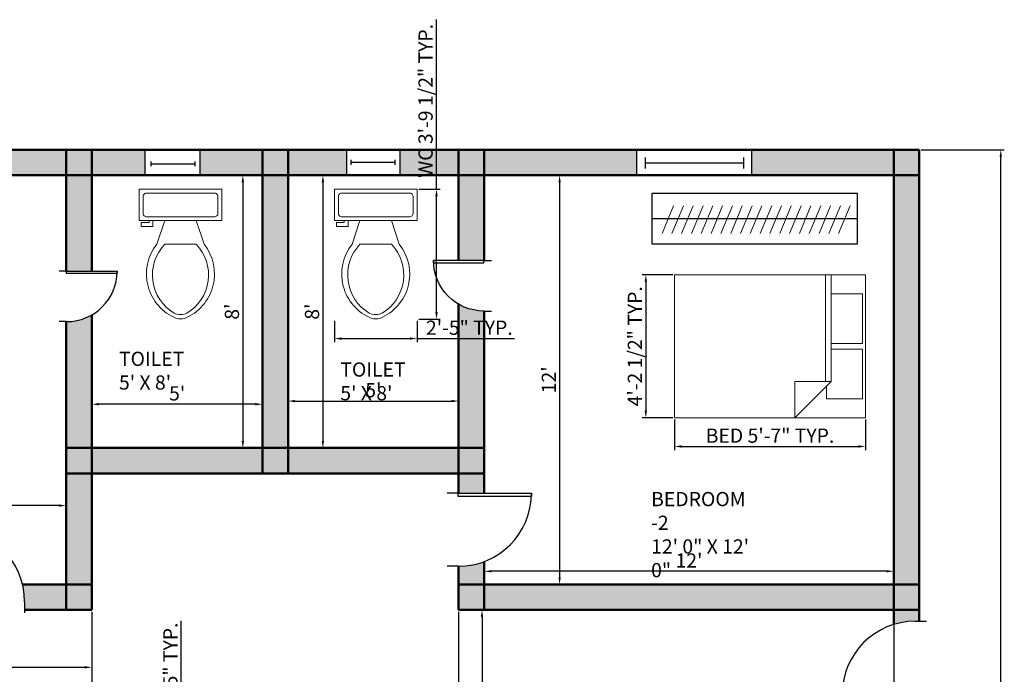
# Model space of a CAD drawing. Units: millimetres. Extents: x 2829 to 4029, y 962 to 1687.
# Tile 4 of 7: x 3053 to 3399, y 1440 to 1670. Entities that reach past the tile are written whole.
import ezdxf

# ---------------------------------------------------------------- set-up
doc = ezdxf.new("R2010")
doc.units = ezdxf.units.MM
for name, color, linetype, lineweight in [('A-ANNO-DIMS', 140, 'Continuous', 18), ('A-AREA-IDEN', 190, 'Continuous', 25), ('A-FLOR-CASE', 90, 'Continuous', 25), ('A-FLOR-CASE-PATT', 90, 'Continuous', 13), ('A-FLOR-FIXT', 90, 'Continuous', 18), ('A-WALL-PATT', 2, 'Continuous', 13), ('doors', 10, 'Continuous', 25), ('furniture', 90, 'Continuous', 18), ('walls', 50, 'Continuous', 50), ('windows', 30, 'Continuous', 25)]:
    doc.layers.add(name, color=color, linetype=linetype, lineweight=lineweight)
doc.styles.get("Standard").update_dxf_attribs({"font": 'arial.ttf'})
doc.dimstyles.new('ISO-25', dxfattribs={"dimtxt": 5, "dimasz": 2.5, "dimexe": 1.25, "dimexo": 0.625, "dimtad": 1, "dimdec": 0, "dimlunit": 3, "dimtxsty": 'Standard', "dimcen": 2.5, "dimadec": 0, "dimazin": 0, "dimtfac": 1, "dimtdec": 0, "dimtmove": 0, "dimatfit": 3, "dimfxl": 1, "dimarcsym": 0})

# ---------------------------------------------------------------- blocks, each defined once
blk = doc.blocks.new('*U2')
for p, q in [((0, 0), (0, -6)), ((40, 0), (40, -6))]:
    blk.add_line(p, q)
blk.add_lwpolyline([(0, 0), (0, 40), (1.75, 40), (1.75, 0)], close=True)
blk.add_arc((0, 0), 40, 0, 90)
blk = doc.blocks.new('*U5')
for p, q in [((0, 4), (0, 0)), ((0, 2), (36, 2)), ((36, 4), (36, 0))]:
    blk.add_line(p, q)
blk = doc.blocks.new('*U4')
for p, q in [((0, 4), (0, 0)), ((36, 4), (36, 0)), ((0, 2), (36, 2))]:
    blk.add_line(p, q)
blk = doc.blocks.new('Bed - Queen')
for p, q in [((0, -80.00003), (0, 0)), ((0, 0), (59.99999, 0)), ((59.99999, 0), (59.99999, -80.00003)), ((7.99999, -1.2), (28.79998, -1.2)), ((7.99999, -14.4), (7.99999, -1.2)), ((28.79998, -1.2), (28.79998, -14.4)), ((31.19999, -1.2), (51.99999, -1.2)), ((31.19999, -14.4), (31.19999, -1.2)), ((51.99999, -1.2), (51.99999, -16.4)), ((0, -14.4), (44.8, -14.4)), ((59.99999, -29.6), (44.8, -14.4)), ((44.8, -14.4), (44.8, -29.6)), ((51.99999, -16.4), (46.79936, -16.4)), ((44.8, -16.8), (0, -16.8)), ((44.8, -29.6), (59.99999, -29.6)), ((59.99999, -80.00003), (0, -80.00003))]:
    blk.add_line(p, q)
blk = doc.blocks.new('Toilet - top')
for p, q in [((9.5, -6), (9.5, -2)), ((-10, -8.5), (-8, -8.5)), ((-10, -9.5), (-10, -8.5)), ((-7, -9.5), (-10, -9.5)), ((-8, -8.5), (-8, -8)), ((-7, -8), (-7, -9.5)), ((-4, -8), (-6, -14)), ((4, -8), (6, -14)), ((4, -14), (-4, -14))]:
    blk.add_line(p, q)
blk.add_lwpolyline([(10.5, -8), (10.5, 0), (-10.5, 0), (-10.5, -8)], close=True)
for points in [[(-9.5, -2), (-9.5, -6)], [(8.5, -1), (-8.5, -1)], [(-8.5, -7), (8.5, -7)]]:
    blk.add_lwpolyline(points)
for centre, radius, start, end in [((-8.62, -1.88), 0.884, 81.8699, 188.1301), ((8.62, -1.88), 0.884, 351.8699, 98.1301), ((-8.62, -6.12), 0.884, 171.8699, 278.1301), ((8.62, -6.12), 0.884, 261.8699, 8.1301), ((3.52, -21.58), 12.17, 141.4691, 247.9714), ((4.2, -21.82), 11.33, 136.3677, 238.9468), ((-3.52, -21.58), 12.17, 292.0284, 38.5307), ((-4.2, -21.82), 11.33, 301.053, 43.6321), ((0, -27.88), 4, 245.7318, 294.2682), ((0, -29), 4, 254.8605, 285.1395)]:
    blk.add_arc(centre, radius, start, end)
blk = doc.blocks.new('*D12')
at = {"layer": 'A-ANNO-DIMS', "color": 0, "lineweight": -2, "transparency": 16777216}
for p, q in [((2937.31, 1499.73), (2937.31, 1500.36)), ((3069.31, 1499.73), (3069.31, 1500.36)), ((3066.81, 1499.11), (2939.81, 1499.11))]:
    blk.add_line(p, q, dxfattribs=at)
at = {"layer": 'A-ANNO-DIMS', "color": 0, "transparency": 16777216}
for points in [[(2939.81, 1499.52), (2939.81, 1498.69), (2937.31, 1499.11)], [(3066.81, 1499.52), (3066.81, 1498.69), (3069.31, 1499.11)]]:
    blk.add_solid(points, dxfattribs=at)
at = {"layer": 'Defpoints', "color": 0, "transparency": 16777216}
for p in [(2937.31, 1499.11), (2937.31, 1499.11), (3069.31, 1499.11)]:
    blk.add_point(p, dxfattribs=at)
at = {"layer": 'A-ANNO-DIMS', "color": 0, "transparency": 16777216, "insert": (3003.31, 1502.24), "char_height": 5, "attachment_point": 5}
blk.add_mtext("11'", dxfattribs=at)
blk = doc.blocks.new('*D13')
at = {"layer": 'A-ANNO-DIMS', "color": 0, "lineweight": -2, "transparency": 16777216}
for p, q in [((3131.71, 1615.38), (3132.65, 1615.38)), ((3131.4, 1612.88), (3131.4, 1521.88)), ((3131.71, 1519.38), (3132.65, 1519.38))]:
    blk.add_line(p, q, dxfattribs=at)
at = {"layer": 'A-ANNO-DIMS', "color": 0, "transparency": 16777216}
for points in [[(3130.98, 1612.88), (3131.82, 1612.88), (3131.4, 1615.38)], [(3130.98, 1521.88), (3131.82, 1521.88), (3131.4, 1519.38)]]:
    blk.add_solid(points, dxfattribs=at)
at = {"layer": 'Defpoints', "color": 0, "transparency": 16777216}
for p in [(3131.09, 1615.38), (3131.09, 1519.38), (3131.4, 1519.38)]:
    blk.add_point(p, dxfattribs=at)
at = {"layer": 'A-ANNO-DIMS', "color": 0, "transparency": 16777216, "insert": (3128.22, 1567.38), "char_height": 5, "attachment_point": 5, "rotation": 90}
blk.add_mtext("8'", dxfattribs=at)
blk = doc.blocks.new('*D14')
at = {"layer": 'A-ANNO-DIMS', "color": 0, "lineweight": -2, "transparency": 16777216}
for p, q in [((3078.31, 1535.41), (3078.31, 1536.04)), ((3135.81, 1534.79), (3080.81, 1534.79)), ((3138.31, 1535.41), (3138.31, 1536.04))]:
    blk.add_line(p, q, dxfattribs=at)
at = {"layer": 'A-ANNO-DIMS', "color": 0, "transparency": 16777216}
for points in [[(3080.81, 1535.2), (3080.81, 1534.37), (3078.31, 1534.79)], [(3135.81, 1535.2), (3135.81, 1534.37), (3138.31, 1534.79)]]:
    blk.add_solid(points, dxfattribs=at)
at = {"layer": 'Defpoints', "color": 0, "transparency": 16777216}
for p in [(3078.31, 1534.79), (3078.31, 1534.79), (3138.31, 1534.79)]:
    blk.add_point(p, dxfattribs=at)
at = {"layer": 'A-ANNO-DIMS', "color": 0, "transparency": 16777216, "insert": (3108.31, 1537.95), "char_height": 5, "attachment_point": 5}
blk.add_mtext("5'", dxfattribs=at)
blk = doc.blocks.new('*D15')
at = {"layer": 'A-ANNO-DIMS', "color": 0, "lineweight": -2, "transparency": 16777216}
for p, q in [((3147.31, 1535.41), (3147.31, 1537.14)), ((3149.81, 1535.89), (3204.81, 1535.89)), ((3207.31, 1535.41), (3207.31, 1537.14))]:
    blk.add_line(p, q, dxfattribs=at)
at = {"layer": 'A-ANNO-DIMS', "color": 0, "transparency": 16777216}
for points in [[(3149.81, 1536.31), (3149.81, 1535.47), (3147.31, 1535.89)], [(3204.81, 1536.31), (3204.81, 1535.47), (3207.31, 1535.89)]]:
    blk.add_solid(points, dxfattribs=at)
at = {"layer": 'Defpoints', "color": 0, "transparency": 16777216}
for p in [(3147.31, 1534.79), (3207.31, 1535.89), (3207.31, 1534.79)]:
    blk.add_point(p, dxfattribs=at)
at = {"layer": 'A-ANNO-DIMS', "color": 0, "transparency": 16777216, "insert": (3177.31, 1539.06), "char_height": 5, "attachment_point": 5}
blk.add_mtext("5'", dxfattribs=at)
blk = doc.blocks.new('*D16')
at = {"layer": 'A-ANNO-DIMS', "color": 0, "lineweight": -2, "transparency": 16777216}
for p, q in [((3155.72, 1615.38), (3160.81, 1615.38)), ((3159.56, 1612.88), (3159.56, 1521.88)), ((3155.72, 1519.38), (3160.81, 1519.38))]:
    blk.add_line(p, q, dxfattribs=at)
at = {"layer": 'A-ANNO-DIMS', "color": 0, "transparency": 16777216}
for points in [[(3159.15, 1612.88), (3159.98, 1612.88), (3159.56, 1615.38)], [(3159.15, 1521.88), (3159.98, 1521.88), (3159.56, 1519.38)]]:
    blk.add_solid(points, dxfattribs=at)
at = {"layer": 'Defpoints', "color": 0, "transparency": 16777216}
for p in [(3155.1, 1615.38), (3155.1, 1519.38), (3159.56, 1519.38)]:
    blk.add_point(p, dxfattribs=at)
at = {"layer": 'A-ANNO-DIMS', "color": 0, "transparency": 16777216, "insert": (3156.39, 1567.38), "char_height": 5, "attachment_point": 5, "rotation": 90}
blk.add_mtext("8'", dxfattribs=at)
blk = doc.blocks.new('*D17')
at = {"layer": 'A-ANNO-DIMS', "color": 0, "lineweight": -2, "transparency": 16777216}
for p, q in [((3360.31, 1480.59), (3360.31, 1474.74)), ((3216.31, 1476.61), (3216.31, 1477.24)), ((3357.81, 1475.99), (3218.81, 1475.99))]:
    blk.add_line(p, q, dxfattribs=at)
at = {"layer": 'A-ANNO-DIMS', "color": 0, "transparency": 16777216}
for points in [[(3218.81, 1476.4), (3218.81, 1475.57), (3216.31, 1475.99)], [(3357.81, 1476.4), (3357.81, 1475.57), (3360.31, 1475.99)]]:
    blk.add_solid(points, dxfattribs=at)
at = {"layer": 'Defpoints', "color": 0, "transparency": 16777216}
for p in [(3360.31, 1481.22), (3216.31, 1475.99), (3216.31, 1475.99)]:
    blk.add_point(p, dxfattribs=at)
at = {"layer": 'A-ANNO-DIMS', "color": 0, "transparency": 16777216, "insert": (3288.31, 1479.12), "char_height": 5, "attachment_point": 5}
blk.add_mtext("12'", dxfattribs=at)
blk = doc.blocks.new('*D18')
at = {"layer": 'A-ANNO-DIMS', "color": 0, "lineweight": -2, "transparency": 16777216}
for p, q in [((3243.44, 1615.38), (3244.06, 1615.38)), ((3242.81, 1612.88), (3242.81, 1473.88)), ((3243.44, 1471.38), (3244.06, 1471.38))]:
    blk.add_line(p, q, dxfattribs=at)
at = {"layer": 'A-ANNO-DIMS', "color": 0, "transparency": 16777216}
for points in [[(3242.4, 1612.88), (3243.23, 1612.88), (3242.81, 1615.38)], [(3242.4, 1473.88), (3243.23, 1473.88), (3242.81, 1471.38)]]:
    blk.add_solid(points, dxfattribs=at)
at = {"layer": 'Defpoints', "color": 0, "transparency": 16777216}
for p in [(3242.81, 1615.38), (3242.81, 1471.38), (3242.81, 1471.38)]:
    blk.add_point(p, dxfattribs=at)
at = {"layer": 'A-ANNO-DIMS', "color": 0, "transparency": 16777216, "insert": (3239.68, 1543.38), "char_height": 5, "attachment_point": 5, "rotation": 90}
blk.add_mtext("12'", dxfattribs=at)
blk = doc.blocks.new('*D27')
at = {"layer": 'A-ANNO-DIMS', "color": 0, "lineweight": -2, "transparency": 16777216}
for p, q in [((2937.31, 1461.76), (2937.31, 1440.93)), ((3078.31, 1461.76), (3078.31, 1440.93)), ((2939.81, 1442.18), (3075.81, 1442.18))]:
    blk.add_line(p, q, dxfattribs=at)
at = {"layer": 'A-ANNO-DIMS', "color": 0, "transparency": 16777216}
for points in [[(2939.81, 1442.59), (2939.81, 1441.76), (2937.31, 1442.18)], [(3075.81, 1442.59), (3075.81, 1441.76), (3078.31, 1442.18)]]:
    blk.add_solid(points, dxfattribs=at)
at = {"layer": 'Defpoints', "color": 0, "transparency": 16777216}
for p in [(2937.31, 1462.38), (3078.31, 1462.38), (3078.31, 1442.18)]:
    blk.add_point(p, dxfattribs=at)
at = {"layer": 'A-ANNO-DIMS', "color": 0, "transparency": 16777216, "insert": (3007.81, 1445.36), "char_height": 5, "attachment_point": 5}
blk.add_mtext('11\'-9"', dxfattribs=at)
blk = doc.blocks.new('*D28')
at = {"layer": 'A-ANNO-DIMS', "color": 0, "lineweight": -2, "transparency": 16777216}
for p, q in [((3215.69, 1462.38), (3214.27, 1462.38)), ((3215.52, 1459.88), (3215.52, 1326.88)), ((3215.69, 1324.38), (3214.27, 1324.38))]:
    blk.add_line(p, q, dxfattribs=at)
at = {"layer": 'A-ANNO-DIMS', "color": 0, "transparency": 16777216}
for points in [[(3215.1, 1459.88), (3215.93, 1459.88), (3215.52, 1462.38)], [(3215.1, 1326.88), (3215.93, 1326.88), (3215.52, 1324.38)]]:
    blk.add_solid(points, dxfattribs=at)
at = {"layer": 'Defpoints', "color": 0, "transparency": 16777216}
for p in [(3216.31, 1462.38), (3215.52, 1324.38), (3216.31, 1324.38)]:
    blk.add_point(p, dxfattribs=at)
at = {"layer": 'A-ANNO-DIMS', "color": 0, "transparency": 16777216, "insert": (3212.34, 1393.38), "char_height": 5, "attachment_point": 5, "rotation": 90}
blk.add_mtext('11\'-6"', dxfattribs=at)
blk = doc.blocks.new('*D29')
at = {"layer": 'A-ANNO-DIMS', "color": 0, "lineweight": -2, "transparency": 16777216}
for p, q in [((3207.31, 1461.76), (3207.31, 1408.16)), ((3360.31, 1461.76), (3360.31, 1408.16)), ((3209.81, 1409.41), (3357.81, 1409.41))]:
    blk.add_line(p, q, dxfattribs=at)
at = {"layer": 'A-ANNO-DIMS', "color": 0, "transparency": 16777216}
for points in [[(3209.81, 1409.83), (3209.81, 1408.99), (3207.31, 1409.41)], [(3357.81, 1409.83), (3357.81, 1408.99), (3360.31, 1409.41)]]:
    blk.add_solid(points, dxfattribs=at)
at = {"layer": 'Defpoints', "color": 0, "transparency": 16777216}
for p in [(3207.31, 1462.38), (3360.31, 1462.38), (3360.31, 1409.41)]:
    blk.add_point(p, dxfattribs=at)
at = {"layer": 'A-ANNO-DIMS', "color": 0, "transparency": 16777216, "insert": (3283.81, 1412.59), "char_height": 5, "attachment_point": 5}
blk.add_mtext('12\'-9"', dxfattribs=at)
blk = doc.blocks.new('*D30')
at = {"layer": 'A-ANNO-DIMS', "color": 0, "lineweight": -2, "transparency": 16777216}
for p, q in [((3078.31, 1461.76), (3078.31, 1406.92)), ((3207.31, 1461.76), (3207.31, 1406.92)), ((3080.81, 1408.17), (3204.81, 1408.17))]:
    blk.add_line(p, q, dxfattribs=at)
at = {"layer": 'A-ANNO-DIMS', "color": 0, "transparency": 16777216}
for points in [[(3080.81, 1408.59), (3080.81, 1407.75), (3078.31, 1408.17)], [(3204.81, 1408.59), (3204.81, 1407.75), (3207.31, 1408.17)]]:
    blk.add_solid(points, dxfattribs=at)
at = {"layer": 'Defpoints', "color": 0, "transparency": 16777216}
for p in [(3078.31, 1462.38), (3207.31, 1462.38), (3207.31, 1408.17)]:
    blk.add_point(p, dxfattribs=at)
at = {"layer": 'A-ANNO-DIMS', "color": 0, "transparency": 16777216, "insert": (3142.81, 1411.35), "char_height": 5, "attachment_point": 5}
blk.add_mtext('10\'-9"', dxfattribs=at)
blk = doc.blocks.new('*D69')
at = {"layer": 'A-ANNO-DIMS', "color": 0, "lineweight": -2, "transparency": 16777216}
for p, q in [((3283.22, 1529.36), (3283.22, 1518.66)), ((3350.4, 1529.36), (3350.4, 1518.66)), ((3285.72, 1519.91), (3347.9, 1519.91))]:
    blk.add_line(p, q, dxfattribs=at)
at = {"layer": 'A-ANNO-DIMS', "color": 0, "transparency": 16777216}
for points in [[(3285.72, 1520.33), (3285.72, 1519.49), (3283.22, 1519.91)], [(3347.9, 1520.33), (3347.9, 1519.49), (3350.4, 1519.91)]]:
    blk.add_solid(points, dxfattribs=at)
at = {"layer": 'Defpoints', "color": 0, "transparency": 16777216}
for p in [(3283.22, 1529.99), (3350.4, 1529.99), (3350.4, 1519.91)]:
    blk.add_point(p, dxfattribs=at)
at = {"layer": 'A-ANNO-DIMS', "color": 0, "transparency": 16777216, "insert": (3316.81, 1523.08), "char_height": 5, "attachment_point": 5}
blk.add_mtext('BED 5\'-7" TYP.', dxfattribs=at)
blk = doc.blocks.new('*D70')
at = {"layer": 'A-ANNO-DIMS', "color": 0, "lineweight": -2, "transparency": 16777216}
for p, q in [((3282.59, 1580.38), (3271.89, 1580.38)), ((3273.14, 1577.88), (3273.14, 1532.49)), ((3282.59, 1529.99), (3271.89, 1529.99))]:
    blk.add_line(p, q, dxfattribs=at)
at = {"layer": 'A-ANNO-DIMS', "color": 0, "transparency": 16777216}
for points in [[(3272.72, 1577.88), (3273.55, 1577.88), (3273.14, 1580.38)], [(3272.72, 1532.49), (3273.55, 1532.49), (3273.14, 1529.99)]]:
    blk.add_solid(points, dxfattribs=at)
at = {"layer": 'Defpoints', "color": 0, "transparency": 16777216}
for p in [(3283.22, 1580.38), (3273.14, 1529.99), (3283.22, 1529.99)]:
    blk.add_point(p, dxfattribs=at)
at = {"layer": 'A-ANNO-DIMS', "color": 0, "transparency": 16777216, "insert": (3269.93, 1555.18), "char_height": 5, "attachment_point": 5, "rotation": 90}
blk.add_mtext('4\'-2 1/2" TYP.', dxfattribs=at)
blk = doc.blocks.new('*D73')
at = {"layer": 'A-ANNO-DIMS', "color": 0, "lineweight": -2, "transparency": 16777216}
for p, q in [((3199.53, 1610.48), (3199.53, 1670.15)), ((3193.29, 1610.48), (3200.78, 1610.48)), ((3199.53, 1567.25), (3199.53, 1607.98)), ((3193.29, 1564.75), (3200.78, 1564.75))]:
    blk.add_line(p, q, dxfattribs=at)
at = {"layer": 'A-ANNO-DIMS', "color": 0, "transparency": 16777216}
for points in [[(3199.11, 1607.98), (3199.94, 1607.98), (3199.53, 1610.48)], [(3199.11, 1567.25), (3199.94, 1567.25), (3199.53, 1564.75)]]:
    blk.add_solid(points, dxfattribs=at)
at = {"layer": 'Defpoints', "color": 0, "transparency": 16777216}
for p in [(3192.67, 1610.48), (3199.53, 1610.48), (3192.67, 1564.75)]:
    blk.add_point(p, dxfattribs=at)
at = {"layer": 'A-ANNO-DIMS', "color": 0, "transparency": 16777216, "insert": (3196.32, 1641.56), "char_height": 5, "attachment_point": 5, "rotation": 90}
blk.add_mtext('WC 3\'-9 1/2" TYP.', dxfattribs=at)
blk = doc.blocks.new('*D74')
at = {"layer": 'A-ANNO-DIMS', "color": 0, "lineweight": -2, "transparency": 16777216}
for p, q in [((3163.61, 1564.13), (3163.61, 1556.64)), ((3192.67, 1564.13), (3192.67, 1556.64)), ((3166.11, 1557.89), (3190.17, 1557.89)), ((3192.67, 1557.89), (3226.98, 1557.89))]:
    blk.add_line(p, q, dxfattribs=at)
at = {"layer": 'A-ANNO-DIMS', "color": 0, "transparency": 16777216}
for points in [[(3166.11, 1558.31), (3166.11, 1557.48), (3163.61, 1557.89)], [(3190.17, 1558.31), (3190.17, 1557.48), (3192.67, 1557.89)]]:
    blk.add_solid(points, dxfattribs=at)
at = {"layer": 'Defpoints', "color": 0, "transparency": 16777216}
for p in [(3163.61, 1564.75), (3192.67, 1564.75), (3192.67, 1557.89)]:
    blk.add_point(p, dxfattribs=at)
at = {"layer": 'A-ANNO-DIMS', "color": 0, "transparency": 16777216, "insert": (3211.07, 1561.07), "char_height": 5, "attachment_point": 5}
blk.add_mtext('2\'-5" TYP.', dxfattribs=at)
blk = doc.blocks.new('*D80')
at = {"layer": 'A-ANNO-DIMS', "color": 0, "lineweight": -2, "transparency": 16777216}
for p, q in [((3109.76, 1424.31), (3109.76, 1458.54)), ((3110.63, 1421.81), (3108.51, 1421.81)), ((3109.76, 1416.81), (3109.76, 1421.81)), ((3110.63, 1416.81), (3108.51, 1416.81)), ((3109.76, 1414.31), (3109.76, 1411.81))]:
    blk.add_line(p, q, dxfattribs=at)
at = {"layer": 'A-ANNO-DIMS', "color": 0, "transparency": 16777216}
for points in [[(3109.34, 1424.31), (3110.17, 1424.31), (3109.76, 1421.81)], [(3109.34, 1414.31), (3110.17, 1414.31), (3109.76, 1416.81)]]:
    blk.add_solid(points, dxfattribs=at)
at = {"layer": 'Defpoints', "color": 0, "transparency": 16777216}
for p in [(3109.76, 1421.81), (3111.25, 1421.81), (3111.25, 1416.81)]:
    blk.add_point(p, dxfattribs=at)
at = {"layer": 'A-ANNO-DIMS', "color": 0, "transparency": 16777216, "insert": (3106.58, 1442.67), "char_height": 5, "attachment_point": 5, "rotation": 90}
blk.add_mtext('0\'-5" TYP.', dxfattribs=at)
blk = doc.blocks.new('*D90')
at = {"layer": 'A-ANNO-DIMS', "color": 0, "lineweight": -2, "transparency": 16777216}
for p, q in [((3369.94, 1624.38), (3399.21, 1624.38)), ((3397.96, 1124.88), (3397.96, 1621.88)), ((3369.94, 1122.38), (3399.21, 1122.38))]:
    blk.add_line(p, q, dxfattribs=at)
at = {"layer": 'A-ANNO-DIMS', "color": 0, "transparency": 16777216}
for points in [[(3397.54, 1621.88), (3398.38, 1621.88), (3397.96, 1624.38)], [(3397.54, 1124.88), (3398.38, 1124.88), (3397.96, 1122.38)]]:
    blk.add_solid(points, dxfattribs=at)
at = {"layer": 'Defpoints', "color": 0, "transparency": 16777216}
for p in [(3369.31, 1624.38), (3397.96, 1624.38), (3369.31, 1122.38)]:
    blk.add_point(p, dxfattribs=at)
at = {"layer": 'A-ANNO-DIMS', "color": 0, "transparency": 16777216, "insert": (3394.78, 1373.38), "char_height": 5, "attachment_point": 5, "rotation": 90}
blk.add_mtext('41\'-10"', dxfattribs=at)

msp = doc.modelspace()

# ---------------------------------------------------------------- hatches: boundary and pattern name
at = {"layer": 'A-FLOR-CASE-PATT'}
h = msp.add_hatch(dxfattribs=at)
h.set_pattern_fill('ANSI31', color=256, scale=1.00365, angle=22.427, style=0)
h.paths.add_polyline_path([(3275.73, 1594.86), (3341.29, 1594.86), (3345.36, 1604.65), (3279.8, 1604.65)])
at = {"layer": 'A-WALL-PATT'}
h = msp.add_hatch(color=256, dxfattribs=at)
h.dxf.hatch_style = 1
h.paths.add_polyline_path([(2969.05, 1624.38), (2937.31, 1624.38), (2937.31, 1615.38), (2969.05, 1615.38)])
h.paths.add_polyline_path([(2937.31, 1624.38), (2928.31, 1624.38), (2928.31, 1615.38), (2937.31, 1615.38)])
h.paths.add_polyline_path([(2937.31, 1615.38), (2928.31, 1615.38), (2928.31, 1471.38), (2937.31, 1471.38)])
h.paths.add_polyline_path([(3069.31, 1624.38), (3011.61, 1624.38), (3011.61, 1615.38), (3069.31, 1615.38)])
h.paths.add_polyline_path([(3078.31, 1624.38), (3069.31, 1624.38), (3069.31, 1615.38), (3078.31, 1615.38)])
h.paths.add_polyline_path([(3078.31, 1615.38), (3069.31, 1615.38), (3069.31, 1581.62), (3069.43, 1581.62), (3078.31, 1581.62)])
h.paths.add_polyline_path([(3078.31, 1566.24, -0.131652), (3069.43, 1563.86), (3069.31, 1563.86), (3069.31, 1519.38), (3078.31, 1519.38)])
h.paths.add_polyline_path([(3078.31, 1519.38), (3069.31, 1519.38), (3069.31, 1510.38), (3078.31, 1510.38)])
h.paths.add_polyline_path([(3138.31, 1519.38), (3078.31, 1519.38), (3078.31, 1510.38), (3138.31, 1510.38)])
h.paths.add_polyline_path([(3147.31, 1519.38), (3138.31, 1519.38), (3138.31, 1510.38), (3147.31, 1510.38)])
h.paths.add_polyline_path([(3147.31, 1615.38), (3138.31, 1615.38), (3138.31, 1519.38), (3147.31, 1519.38)])
h.paths.add_polyline_path([(3147.31, 1624.38), (3138.31, 1624.38), (3138.31, 1615.38), (3147.31, 1615.38)])
h.paths.add_polyline_path([(3138.31, 1624.38), (3116.25, 1624.38), (3116.25, 1615.38), (3138.31, 1615.38)])
h.paths.add_polyline_path([(3096.9, 1624.38), (3078.31, 1624.38), (3078.31, 1615.38), (3096.9, 1615.38)])
h.paths.add_polyline_path([(3167.88, 1624.38), (3147.31, 1624.38), (3147.31, 1615.38), (3167.88, 1615.38)])
h.paths.add_polyline_path([(3207.31, 1624.38), (3186.66, 1624.38), (3186.66, 1615.38), (3207.31, 1615.38)])
h.paths.add_polyline_path([(3216.31, 1624.38), (3207.31, 1624.38), (3207.31, 1615.38), (3216.31, 1615.38)])
h.paths.add_polyline_path([(3216.31, 1615.38), (3207.31, 1615.38), (3207.31, 1585.36), (3216.31, 1585.36)])
h.paths.add_polyline_path([(3216.31, 1567.6), (3216.21, 1567.6, -0.131958), (3207.31, 1569.99), (3207.31, 1519.38), (3216.31, 1519.38)])
h.paths.add_polyline_path([(3216.31, 1519.38), (3207.31, 1519.38), (3207.31, 1510.38), (3216.31, 1510.38)])
h.paths.add_polyline_path([(3207.31, 1519.38), (3147.31, 1519.38), (3147.31, 1510.38), (3207.31, 1510.38)])
h.paths.add_polyline_path([(3269.97, 1624.38), (3216.31, 1624.38), (3216.31, 1615.38), (3269.97, 1615.38)])
h.paths.add_polyline_path([(3360.31, 1624.38), (3310.37, 1624.38), (3310.37, 1615.38), (3360.31, 1615.38)])
h.paths.add_polyline_path([(3369.31, 1624.38), (3360.31, 1624.38), (3360.31, 1615.38), (3369.31, 1615.38)])
h.paths.add_polyline_path([(3369.31, 1615.38), (3360.31, 1615.38), (3360.31, 1471.38), (3369.31, 1471.38)])
h.paths.add_polyline_path([(3360.31, 1471.38), (3216.31, 1471.38), (3216.31, 1462.38), (3360.31, 1462.38)])
h.paths.add_polyline_path([(3216.31, 1471.38), (3207.31, 1471.38), (3207.31, 1462.38), (3216.31, 1462.38)])
h.paths.add_polyline_path([(3216.31, 1479.42, -0.089587), (3207.31, 1477.74), (3207.31, 1471.38), (3216.31, 1471.38)])
h.paths.add_polyline_path([(3216.31, 1510.38), (3207.31, 1510.38), (3207.31, 1503.49), (3216.31, 1503.49)])
h.paths.add_polyline_path([(3369.31, 1471.38), (3360.31, 1471.38), (3360.31, 1462.38), (3369.31, 1462.38)])
h.paths.add_polyline_path([(3360.31, 1324.38), (3163.31, 1324.38), (3163.31, 1315.38), (3360.31, 1315.38)])
h.paths.add_polyline_path([(3369.31, 1324.38), (3360.31, 1324.38), (3360.31, 1315.38), (3369.31, 1315.38)])
h.paths.add_polyline_path([(3028.89, 1471.38), (2937.31, 1471.38), (2937.31, 1462.38), (3028.89, 1462.38), (3028.89, 1465.26)])
h.paths.add_polyline_path([(2937.31, 1471.38), (2928.31, 1471.38), (2928.31, 1462.38), (2937.31, 1462.38)])
h.paths.add_polyline_path([(2928.31, 1471.38), (2862.31, 1471.38), (2862.31, 1462.38), (2928.31, 1462.38)])
h.paths.add_polyline_path([(2862.31, 1462.38), (2853.31, 1462.38), (2853.31, 1324.38), (2862.31, 1324.38)])
h.paths.add_polyline_path([(2862.31, 1471.38), (2853.31, 1471.38), (2853.31, 1462.38), (2862.31, 1462.38)])
h.paths.add_polyline_path([(2928.31, 1324.38), (2862.31, 1324.38), (2862.31, 1315.38), (2928.31, 1315.38)])
h.paths.add_polyline_path([(2862.31, 1324.38), (2853.31, 1324.38), (2853.31, 1315.38), (2862.31, 1315.38)])
h.paths.add_polyline_path([(3051.08, 1322.02), (3051.08, 1324.38), (2937.31, 1324.38), (2937.31, 1315.38), (3051.95, 1315.38, -0.065323)])
h.paths.add_polyline_path([(2937.31, 1324.38), (2928.31, 1324.38), (2928.31, 1315.38), (2937.31, 1315.38)])
h.paths.add_polyline_path([(3103.31, 1315.38), (3094.31, 1315.38), (3094.31, 1248.38), (3103.31, 1248.38)])
h.paths.add_polyline_path([(3103.31, 1324.38), (3094.31, 1324.38), (3094.31, 1315.38), (3103.31, 1315.38)])
h.paths.add_polyline_path([(3094.31, 1324.38), (3076.83, 1324.38), (3076.83, 1322.02), (3076.83, 1315.38), (3094.31, 1315.38)])
h.paths.add_polyline_path([(3078.31, 1510.38), (3069.31, 1510.38), (3069.31, 1471.38), (3078.31, 1471.38)])
h.paths.add_polyline_path([(3078.31, 1471.38), (3069.31, 1471.38), (3069.31, 1462.38), (3078.31, 1462.38)])
h.paths.add_polyline_path([(3069.31, 1471.38), (3053.91, 1471.38, -0.060076), (3054.65, 1465.26), (3054.65, 1462.38), (3069.31, 1462.38)])
h.paths.add_polyline_path([(2937.31, 1315.38), (2928.31, 1315.38), (2928.31, 1131.38), (2937.31, 1131.38)])
h.paths.add_polyline_path([(2937.31, 1131.38), (2928.31, 1131.38), (2928.31, 1122.38), (2937.31, 1122.38)])
h.paths.add_polyline_path([(2978.9, 1131.38), (2937.31, 1131.38), (2937.31, 1122.38), (2978.9, 1122.38)])
h.paths.add_polyline_path([(3094.31, 1131.38), (3017.24, 1131.38), (3017.24, 1122.38), (3094.31, 1122.38)])
h.paths.add_polyline_path([(3103.31, 1131.38), (3094.31, 1131.38), (3094.31, 1122.38), (3103.31, 1122.38)])
h.paths.add_polyline_path([(3103.31, 1179.58, -0.112378), (3095.63, 1177.83), (3094.31, 1177.83), (3094.31, 1131.38), (3103.31, 1131.38)])
h.paths.add_polyline_path([(3103.31, 1239.38), (3094.31, 1239.38), (3094.31, 1195.59), (3095.63, 1195.59), (3103.31, 1195.59)])
h.paths.add_polyline_path([(3103.31, 1248.38), (3094.31, 1248.38), (3094.31, 1239.38), (3103.31, 1239.38)])
h.paths.add_polyline_path([(3163.31, 1248.38), (3103.31, 1248.38), (3103.31, 1239.38), (3163.31, 1239.38)])
h.paths.add_polyline_path([(3172.31, 1248.38), (3163.31, 1248.38), (3163.31, 1239.38), (3172.31, 1239.38)])
h.paths.add_polyline_path([(3172.31, 1239.38), (3163.31, 1239.38), (3163.31, 1197.38), (3172.31, 1197.38)])
h.paths.add_polyline_path([(3172.31, 1197.38), (3163.31, 1197.38), (3163.31, 1188.38), (3172.31, 1188.38)])
h.paths.add_polyline_path([(3172.31, 1188.38), (3163.31, 1188.38), (3163.31, 1131.38), (3172.31, 1131.38)])
h.paths.add_polyline_path([(3172.31, 1131.38), (3163.31, 1131.38), (3163.31, 1122.38), (3172.31, 1122.38)])
h.paths.add_polyline_path([(3163.31, 1131.38), (3143.05, 1131.38), (3143.05, 1122.38), (3163.31, 1122.38)])
h.paths.add_polyline_path([(3123.82, 1131.38), (3103.31, 1131.38), (3103.31, 1122.38), (3123.82, 1122.38)])
h.paths.add_polyline_path([(3273.8, 1131.38), (3172.31, 1131.38), (3172.31, 1122.38), (3273.8, 1122.38)])
h.paths.add_polyline_path([(3360.31, 1131.38), (3293.49, 1131.38), (3293.49, 1122.38), (3360.31, 1122.38)])
h.paths.add_polyline_path([(3369.31, 1131.38), (3360.31, 1131.38), (3360.31, 1122.38), (3369.31, 1122.38)])
h.paths.add_polyline_path([(3369.31, 1188.38), (3360.31, 1188.38), (3360.31, 1131.38), (3369.31, 1131.38)])
h.paths.add_polyline_path([(3369.31, 1197.38), (3360.31, 1197.38), (3360.31, 1188.38), (3369.31, 1188.38)])
h.paths.add_polyline_path([(3360.31, 1197.38), (3252.19, 1197.38), (3252.19, 1188.38), (3360.31, 1188.38)])
h.paths.add_polyline_path([(3234.43, 1197.38), (3172.31, 1197.38), (3172.31, 1188.38), (3237.05, 1188.38, -0.134312)])
h.paths.add_polyline_path([(3369.31, 1315.38), (3360.31, 1315.38), (3360.31, 1197.38), (3369.31, 1197.38)])
edge = h.paths.add_edge_path()
edge.add_arc((3367.95, 1432.65), 25.75, 90, 107.2357)
edge.add_line((3360.31, 1457.25), (3360.31, 1462.38))
edge.add_line((3360.31, 1462.38), (3369.31, 1462.38))
edge.add_line((3369.31, 1462.38), (3369.31, 1458.41))
edge.add_line((3369.31, 1458.41), (3367.95, 1458.41))
h.paths.add_polyline_path([(3369.31, 1432.65), (3360.31, 1432.65), (3360.31, 1324.38), (3369.31, 1324.38)])

# ---------------------------------------------------------------- linework, layer by layer
at = {"layer": 'A-FLOR-CASE'}
msp.add_line((3347.54, 1600.07), (3275.21, 1600.07), dxfattribs=at)
msp.add_lwpolyline([(3347.54, 1608.94), (3275.21, 1608.94), (3275.21, 1591.21), (3347.54, 1591.21)], close=True, dxfattribs=at)
at = {"layer": 'walls'}
for p, q in [((2928.31, 1624.38), (3369.31, 1624.38)), ((3069.31, 1624.38), (3069.31, 1581.62)), ((3078.31, 1624.38), (3078.31, 1581.62)), ((3138.31, 1624.38), (3138.31, 1510.38)), ((3147.31, 1624.38), (3147.31, 1510.38)), ((3207.31, 1624.38), (3207.31, 1585.36)), ((3216.31, 1624.38), (3216.31, 1585.36)), ((3360.31, 1624.38), (3360.31, 1457.25)), ((3369.31, 1624.38), (3369.31, 1458.41)), ((2928.31, 1615.38), (3369.31, 1615.38)), ((3207.31, 1569.99), (3207.31, 1503.49)), ((3078.31, 1566.24), (3078.31, 1462.38)), ((3216.31, 1567.6), (3216.31, 1503.49)), ((3069.31, 1563.86), (3069.31, 1462.38)), ((3069.31, 1519.38), (3147.31, 1519.38)), ((3069.31, 1519.38), (3216.31, 1519.38)), ((3069.31, 1510.38), (3147.31, 1510.38)), ((3069.31, 1510.38), (3216.31, 1510.38)), ((3216.31, 1479.42), (3216.31, 1462.38)), ((3207.31, 1477.74), (3207.31, 1462.38)), ((3053.91, 1471.38), (3078.31, 1471.38)), ((3053.91, 1471.38), (3078.31, 1471.38)), ((3207.31, 1471.38), (3369.31, 1471.38)), ((3054.65, 1462.38), (3078.31, 1462.38)), ((3054.65, 1462.38), (3078.31, 1462.38)), ((3207.31, 1462.38), (3369.31, 1462.38))]:
    msp.add_line(p, q, dxfattribs=at)
at = {"layer": 'windows'}
for p, q in [((3096.9, 1624.38), (3096.9, 1615.38)), ((3116.25, 1624.38), (3116.25, 1615.38)), ((3167.88, 1624.38), (3167.88, 1615.38)), ((3186.66, 1624.38), (3186.66, 1615.38)), ((3269.97, 1615.38), (3269.97, 1624.38)), ((3310.37, 1615.38), (3310.37, 1624.38))]:
    msp.add_line(p, q, dxfattribs=at)

# ---------------------------------------------------------------- block references
at = {"layer": 'A-FLOR-FIXT', "xscale": 1.383864873127667, "yscale": 1.383864873127667, "zscale": 1.383864873127667}
for p in [(3109.48, 1610.48), (3178.14, 1610.48)]:
    msp.add_blockref('Toilet - top', p, dxfattribs=at)
at = {"layer": 'doors'}
for p, xscale, yscale, zscale, rotation in [((3216.21, 1585.36), -0.4440322775658344, 0.4440322775658344, 0.4440322775658344, 90), ((3069.43, 1581.62), 0.4440322775658344, 0.4440322775658344, 0.4440322775658344, 270), ((3207.16, 1503.49), 0.6438655246665308, 0.6438655246665308, 0.6438655246665308, 270), ((3367.95, 1432.65), 0.6438655246665308, 0.6438655246665308, 0.6438655246665308, 90)]:
    msp.add_blockref('*U2', p, dxfattribs=dict(at, xscale=xscale, yscale=yscale, zscale=zscale, rotation=rotation))
at = {"layer": 'doors', "xscale": 0.6438655246665308, "yscale": 0.6438655246665308, "zscale": 0.6438655246665308}
msp.add_blockref('*U2', (3028.89, 1465.26), dxfattribs=at)
at = {"layer": 'furniture', "xscale": 0.8398385143789401, "yscale": 0.8398385143789401, "zscale": 0.8398385143789401, "rotation": 270}
msp.add_blockref('Bed - Queen', (3350.4, 1580.38), dxfattribs=at)
at = {"layer": 'windows'}
for name, p, xscale, yscale, zscale in [('*U5', (3169.36, 1619.1), 0.4296922913741178, 0.4296922913741178, 0.4296922913741178), ('*U4', (3272.96, 1617.78), 0.9597059461553321, 0.9597059461553321, 0.9597059461553321), ('*U5', (3099.06, 1618.56), 0.4296922913741178, 0.4296922913741178, 0.4296922913741178)]:
    msp.add_blockref(name, p, dxfattribs=dict(at, xscale=xscale, yscale=yscale, zscale=zscale))

# ---------------------------------------------------------------- texts
at = {"layer": 'A-AREA-IDEN', "char_height": 5, "attachment_point": 1}
for s, width, insert in [("TOILET \\P5' X 8'", 32.901, (3087.85, 1553.27)), ("TOILET \\P5' X 8'", 26.3387, (3165.69, 1549.5)), ('BEDROOM -2 \\P12\' 0" X 12\' 0"', 40.2781, (3275, 1503.89))]:
    msp.add_mtext_dynamic_manual_height_columns(s, width=width, gutter_width=12.5, heights=[0], dxfattribs=dict(at, insert=insert))

# ---------------------------------------------------------------- dimensions: what is measured, and where the dimension line sits
at = {"layer": 'A-ANNO-DIMS'}
for base, p1, p2, angle, text, picture, middle in [((3199.53, 1610.48), (3192.67, 1564.75), (3192.67, 1610.48), 90, 'WC <> TYP.', '*D73', (3196.32, 1641.56)), ((3273.14, 1529.99), (3283.22, 1580.38), (3283.22, 1529.99), 270, '<> TYP.', '*D70', (3269.93, 1555.18)), ((3109.76, 1421.81), (3111.25, 1416.81), (3111.25, 1421.81), 90, '<> TYP.', '*D80', (3106.58, 1442.67))]:
    dim = msp.add_linear_dim(base=base, p1=p1, p2=p2, angle=angle, text=text, dimstyle='ISO-25', override={"dimdec": 1, "dimlfac": 1, "dimrnd": 0, "dimzin": 1, "dimdsep": 46, "dimlunit": 4, "dimfrac": 2}, dxfattribs=at)
    dim.commit()
    dim.dimension.update_dxf_attribs({"geometry": picture, "text_midpoint": middle})
for base, p1, p2, override, picture, middle in [((3397.96, 1624.38), (3369.31, 1122.38), (3369.31, 1624.38), {"dimdec": 1, "dimlfac": 1, "dimrnd": 0, "dimzin": 1, "dimdsep": 46, "dimlunit": 4, "dimfrac": 2}, '*D90', (3394.78, 1373.38)), ((3131.4, 1519.38), (3131.09, 1615.38), (3131.09, 1519.38), {"dimclrd": 0, "dimclre": 0, "dimclrt": 0}, '*D13', (3128.22, 1567.38)), ((3159.56, 1519.38), (3155.1, 1615.38), (3155.1, 1519.38), {"dimclrd": 0, "dimclre": 0, "dimclrt": 0}, '*D16', (3156.39, 1567.38)), ((3242.81, 1471.38), (3242.81, 1615.38), (3242.81, 1471.38), {"dimclrd": 0, "dimclre": 0, "dimclrt": 0}, '*D18', (3239.68, 1543.38)), ((3215.52, 1324.38), (3216.31, 1462.38), (3216.31, 1324.38), {"dimclrd": 0, "dimclre": 0, "dimclrt": 0}, '*D28', (3212.34, 1393.38))]:
    dim = msp.add_linear_dim(base=base, p1=p1, p2=p2, angle=90, dimstyle='ISO-25', override=override, dxfattribs=at)
    dim.commit()
    dim.dimension.update_dxf_attribs({"geometry": picture, "text_midpoint": middle})
for base, p1, p2, text, picture, middle in [((3192.67, 1557.89), (3163.61, 1564.75), (3192.67, 1564.75), '<> TYP.', '*D74', (3211.07, 1561.07)), ((3350.4, 1519.91), (3283.22, 1529.99), (3350.4, 1529.99), 'BED <> TYP.', '*D69', (3316.81, 1523.08))]:
    dim = msp.add_linear_dim(base=base, p1=p1, p2=p2, text=text, dimstyle='ISO-25', override={"dimdec": 1, "dimlfac": 1, "dimrnd": 0, "dimzin": 1, "dimdsep": 46, "dimlunit": 4, "dimfrac": 2}, dxfattribs=at)
    dim.commit()
    dim.dimension.update_dxf_attribs({"geometry": picture, "text_midpoint": middle})
for base, p1, p2, picture, middle in [((3078.31, 1534.79), (3138.31, 1534.79), (3078.31, 1534.79), '*D14', (3108.31, 1537.95)), ((3207.31, 1535.89), (3147.31, 1534.79), (3207.31, 1534.79), '*D15', (3177.31, 1539.06)), ((2937.31, 1499.11), (3069.31, 1499.11), (2937.31, 1499.11), '*D12', (3003.31, 1502.24)), ((3216.31, 1475.99), (3360.31, 1481.22), (3216.31, 1475.99), '*D17', (3288.31, 1479.12)), ((3078.31, 1442.18), (2937.31, 1462.38), (3078.31, 1462.38), '*D27', (3007.81, 1445.36)), ((3207.31, 1408.17), (3078.31, 1462.38), (3207.31, 1462.38), '*D30', (3142.81, 1411.35)), ((3360.31, 1409.41), (3207.31, 1462.38), (3360.31, 1462.38), '*D29', (3283.81, 1412.59))]:
    dim = msp.add_linear_dim(base=base, p1=p1, p2=p2, dimstyle='ISO-25', override={"dimclrd": 0, "dimclre": 0, "dimclrt": 0}, dxfattribs=at)
    dim.commit()
    dim.dimension.update_dxf_attribs({"geometry": picture, "text_midpoint": middle})

doc.saveas('drawing.dxf')
